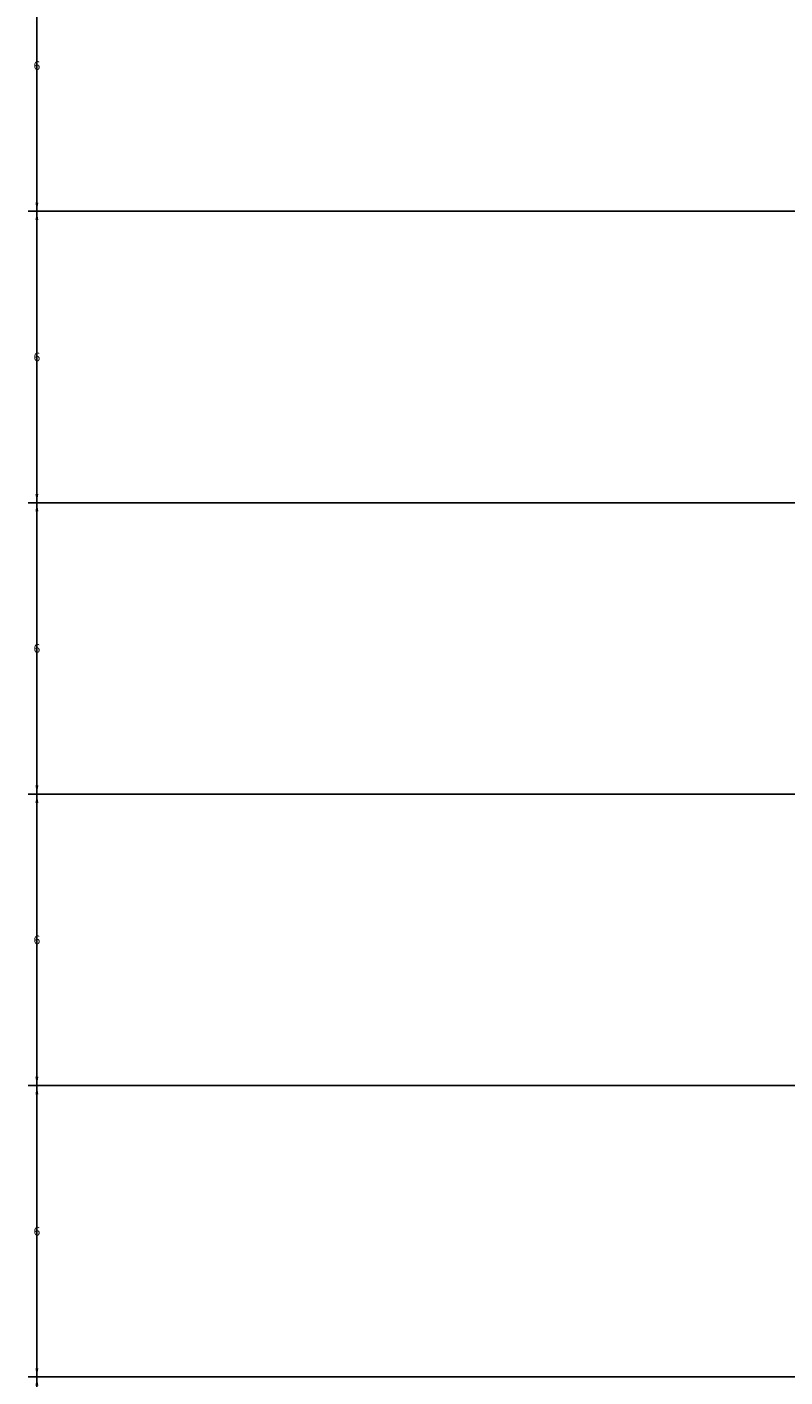
# Model space of a CAD drawing. Units: feet. Extents: x 2695 to 2912, y 795 to 1139.
# Tile 40 of 83: x 2695 to 2710, y 993 to 1020. Entities that reach past the tile are written whole.
import ezdxf

# ---------------------------------------------------------------- set-up
doc = ezdxf.new("R2010")
doc.units = ezdxf.units.FT
doc.layers.add('A-ANNO-DIMS', color=2, linetype='Continuous', lineweight=18)
doc.styles.get("Standard").update_dxf_attribs({"font": 'arial.ttf'})
doc.dimstyles.get("Standard").update_dxf_attribs({"dimtxt": 0.18, "dimasz": 0.18, "dimexe": 0.18, "dimexo": 0.0625, "dimgap": 0.09, "dimtad": 0, "dimtih": 1, "dimtoh": 1, "dimdec": 1, "dimzin": 0, "dimdsep": 46, "dimlunit": 3, "dimtxsty": 'Standard', "dimcen": 0.09, "dimadec": 0, "dimazin": 0, "dimtfac": 1, "dimtdec": 1, "dimtofl": 0, "dimtmove": 0, "dimatfit": 3, "dimfxl": 1, "dimtolj": 1, "dimtzin": 0, "dimarcsym": 0})

# ---------------------------------------------------------------- blocks, each defined once
blk = doc.blocks.new('*D12')
at = {"layer": 'A-ANNO-DIMS', "color": 0, "lineweight": -2, "transparency": 16777216}
for p, q in [((2710.574, 1122.931), (2694.681, 1122.931)), ((2694.861, 1122.751), (2694.861, 967.113)), ((2694.861, 811.111), (2694.861, 966.749)), ((2710.574, 810.931), (2694.681, 810.931))]:
    blk.add_line(p, q, dxfattribs=at)
at = {"layer": 'A-ANNO-DIMS', "color": 0, "transparency": 16777216}
for points in [[(2694.831, 1122.751), (2694.891, 1122.751), (2694.861, 1122.931)], [(2694.831, 811.111), (2694.891, 811.111), (2694.861, 810.931)]]:
    blk.add_solid(points, dxfattribs=at)
at = {"layer": 'Defpoints', "color": 0, "transparency": 16777216}
for p in [(2694.861, 1122.931), (2710.636, 1122.931), (2710.636, 810.931)]:
    blk.add_point(p, dxfattribs=at)
at = {"layer": 'A-ANNO-DIMS', "color": 0, "transparency": 16777216, "insert": (2694.861, 966.931), "char_height": 0.18, "attachment_point": 5}
blk.add_mtext('\\A1;312', dxfattribs=at)
blk = doc.blocks.new('*D36')
at = {"layer": 'A-ANNO-DIMS', "color": 0, "lineweight": -2, "transparency": 16777216}
for p, q in [((2730.646, 992.518), (2694.681, 992.518)), ((2694.861, 992.338), (2694.861, 989.7)), ((2694.861, 986.698), (2694.861, 989.336)), ((2730.646, 986.518), (2694.681, 986.518))]:
    blk.add_line(p, q, dxfattribs=at)
at = {"layer": 'A-ANNO-DIMS', "color": 0, "transparency": 16777216}
for points in [[(2694.831, 992.338), (2694.891, 992.338), (2694.861, 992.518)], [(2694.831, 986.698), (2694.891, 986.698), (2694.861, 986.518)]]:
    blk.add_solid(points, dxfattribs=at)
at = {"layer": 'Defpoints', "color": 0, "transparency": 16777216}
for p in [(2694.861, 992.518), (2730.708, 992.518), (2730.708, 986.518)]:
    blk.add_point(p, dxfattribs=at)
at = {"layer": 'A-ANNO-DIMS', "color": 0, "transparency": 16777216, "insert": (2694.861, 989.518), "char_height": 0.18, "attachment_point": 5}
blk.add_mtext('\\A1;6', dxfattribs=at)
blk = doc.blocks.new('*D37')
at = {"layer": 'A-ANNO-DIMS', "color": 0, "lineweight": -2, "transparency": 16777216}
for p, q in [((2730.646, 998.518), (2694.681, 998.518)), ((2694.861, 998.338), (2694.861, 995.7)), ((2694.861, 992.698), (2694.861, 995.336)), ((2730.646, 992.518), (2694.681, 992.518))]:
    blk.add_line(p, q, dxfattribs=at)
at = {"layer": 'A-ANNO-DIMS', "color": 0, "transparency": 16777216}
for points in [[(2694.831, 998.338), (2694.891, 998.338), (2694.861, 998.518)], [(2694.831, 992.698), (2694.891, 992.698), (2694.861, 992.518)]]:
    blk.add_solid(points, dxfattribs=at)
at = {"layer": 'Defpoints', "color": 0, "transparency": 16777216}
for p in [(2694.861, 998.518), (2730.708, 998.518), (2730.708, 992.518)]:
    blk.add_point(p, dxfattribs=at)
at = {"layer": 'A-ANNO-DIMS', "color": 0, "transparency": 16777216, "insert": (2694.861, 995.518), "char_height": 0.18, "attachment_point": 5}
blk.add_mtext('\\A1;6', dxfattribs=at)
blk = doc.blocks.new('*D38')
at = {"layer": 'A-ANNO-DIMS', "color": 0, "lineweight": -2, "transparency": 16777216}
for p, q in [((2730.646, 1004.518), (2694.681, 1004.518)), ((2694.861, 1004.338), (2694.861, 1001.7)), ((2694.861, 998.698), (2694.861, 1001.336)), ((2730.646, 998.518), (2694.681, 998.518))]:
    blk.add_line(p, q, dxfattribs=at)
at = {"layer": 'A-ANNO-DIMS', "color": 0, "transparency": 16777216}
for points in [[(2694.831, 1004.338), (2694.891, 1004.338), (2694.861, 1004.518)], [(2694.831, 998.698), (2694.891, 998.698), (2694.861, 998.518)]]:
    blk.add_solid(points, dxfattribs=at)
at = {"layer": 'Defpoints', "color": 0, "transparency": 16777216}
for p in [(2694.861, 1004.518), (2730.708, 1004.518), (2730.708, 998.518)]:
    blk.add_point(p, dxfattribs=at)
at = {"layer": 'A-ANNO-DIMS', "color": 0, "transparency": 16777216, "insert": (2694.861, 1001.518), "char_height": 0.18, "attachment_point": 5}
blk.add_mtext('\\A1;6', dxfattribs=at)
blk = doc.blocks.new('*D39')
at = {"layer": 'A-ANNO-DIMS', "color": 0, "lineweight": -2, "transparency": 16777216}
for p, q in [((2730.646, 1010.518), (2694.681, 1010.518)), ((2694.861, 1010.338), (2694.861, 1007.7)), ((2694.861, 1004.698), (2694.861, 1007.336)), ((2730.646, 1004.518), (2694.681, 1004.518))]:
    blk.add_line(p, q, dxfattribs=at)
at = {"layer": 'A-ANNO-DIMS', "color": 0, "transparency": 16777216}
for points in [[(2694.831, 1010.338), (2694.891, 1010.338), (2694.861, 1010.518)], [(2694.831, 1004.698), (2694.891, 1004.698), (2694.861, 1004.518)]]:
    blk.add_solid(points, dxfattribs=at)
at = {"layer": 'Defpoints', "color": 0, "transparency": 16777216}
for p in [(2694.861, 1010.518), (2730.708, 1010.518), (2730.708, 1004.518)]:
    blk.add_point(p, dxfattribs=at)
at = {"layer": 'A-ANNO-DIMS', "color": 0, "transparency": 16777216, "insert": (2694.861, 1007.518), "char_height": 0.18, "attachment_point": 5}
blk.add_mtext('\\A1;6', dxfattribs=at)
blk = doc.blocks.new('*D40')
at = {"layer": 'A-ANNO-DIMS', "color": 0, "lineweight": -2, "transparency": 16777216}
for p, q in [((2730.646, 1016.518), (2694.681, 1016.518)), ((2694.861, 1016.338), (2694.861, 1013.7)), ((2694.861, 1010.698), (2694.861, 1013.336)), ((2730.646, 1010.518), (2694.681, 1010.518))]:
    blk.add_line(p, q, dxfattribs=at)
at = {"layer": 'A-ANNO-DIMS', "color": 0, "transparency": 16777216}
for points in [[(2694.831, 1016.338), (2694.891, 1016.338), (2694.861, 1016.518)], [(2694.831, 1010.698), (2694.891, 1010.698), (2694.861, 1010.518)]]:
    blk.add_solid(points, dxfattribs=at)
at = {"layer": 'Defpoints', "color": 0, "transparency": 16777216}
for p in [(2694.861, 1016.518), (2730.708, 1016.518), (2730.708, 1010.518)]:
    blk.add_point(p, dxfattribs=at)
at = {"layer": 'A-ANNO-DIMS', "color": 0, "transparency": 16777216, "insert": (2694.861, 1013.518), "char_height": 0.18, "attachment_point": 5}
blk.add_mtext('\\A1;6', dxfattribs=at)
blk = doc.blocks.new('*D41')
at = {"layer": 'A-ANNO-DIMS', "color": 0, "lineweight": -2, "transparency": 16777216}
for p, q in [((2730.646, 1022.518), (2694.681, 1022.518)), ((2694.861, 1022.338), (2694.861, 1019.7)), ((2694.861, 1016.698), (2694.861, 1019.336)), ((2730.646, 1016.518), (2694.681, 1016.518))]:
    blk.add_line(p, q, dxfattribs=at)
at = {"layer": 'A-ANNO-DIMS', "color": 0, "transparency": 16777216}
for points in [[(2694.831, 1022.338), (2694.891, 1022.338), (2694.861, 1022.518)], [(2694.831, 1016.698), (2694.891, 1016.698), (2694.861, 1016.518)]]:
    blk.add_solid(points, dxfattribs=at)
at = {"layer": 'Defpoints', "color": 0, "transparency": 16777216}
for p in [(2694.861, 1022.518), (2730.708, 1022.518), (2730.708, 1016.518)]:
    blk.add_point(p, dxfattribs=at)
at = {"layer": 'A-ANNO-DIMS', "color": 0, "transparency": 16777216, "insert": (2694.861, 1019.518), "char_height": 0.18, "attachment_point": 5}
blk.add_mtext('\\A1;6', dxfattribs=at)

msp = doc.modelspace()

# ---------------------------------------------------------------- dimensions: what is measured, and where the dimension line sits
at = {"layer": 'A-ANNO-DIMS'}
for base, p1, p2, picture, middle in [((2694.8611, 1122.9306), (2710.6361, 810.9306), (2710.6361, 1122.9306), '*D12', (2694.8611, 966.9306)), ((2694.8611, 1022.5179), (2730.7081, 1016.5179), (2730.7081, 1022.5179), '*D41', (2694.8611, 1019.5179)), ((2694.8611, 1016.5179), (2730.7081, 1010.5179), (2730.7081, 1016.5179), '*D40', (2694.8611, 1013.5179)), ((2694.8611, 1010.5179), (2730.7081, 1004.5179), (2730.7081, 1010.5179), '*D39', (2694.8611, 1007.5179)), ((2694.8611, 1004.5179), (2730.7081, 998.5179), (2730.7081, 1004.5179), '*D38', (2694.8611, 1001.5179)), ((2694.8611, 998.5179), (2730.7081, 992.5179), (2730.7081, 998.5179), '*D37', (2694.8611, 995.5179)), ((2694.8611, 992.5179), (2730.7081, 986.5179), (2730.7081, 992.5179), '*D36', (2694.8611, 989.5179))]:
    dim = msp.add_linear_dim(base=base, p1=p1, p2=p2, angle=90, dimstyle='Standard', override={"dimdec": 0, "dimlfac": 1, "dimrnd": 0, "dimzin": 0, "dimdsep": 46, "dimlunit": 2}, dxfattribs=at)
    dim.commit()
    dim.dimension.update_dxf_attribs({"geometry": picture, "text_midpoint": middle})

doc.saveas('drawing.dxf')
